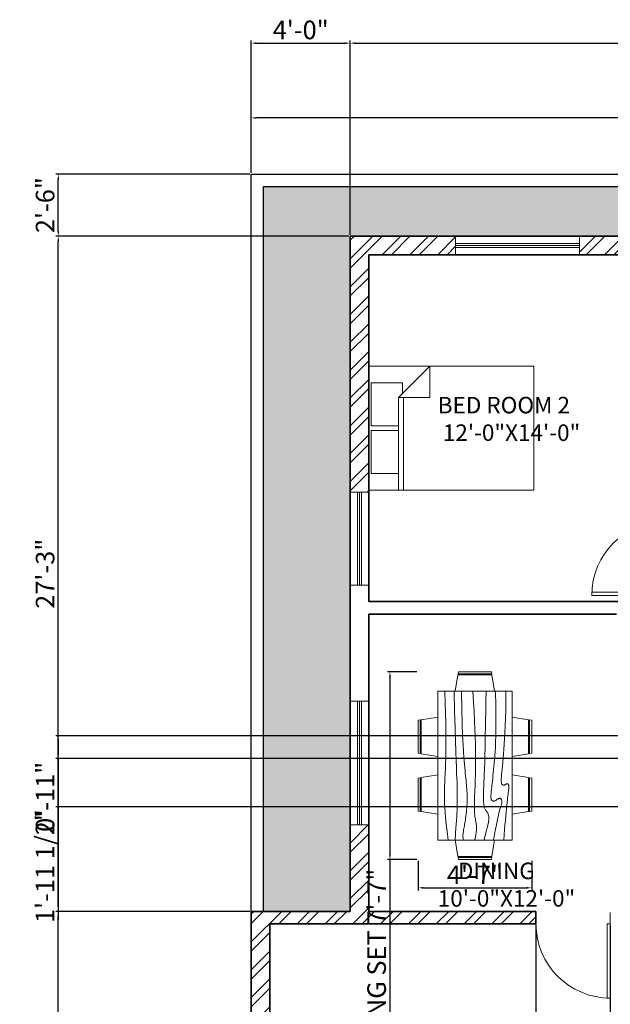
# Model space of a CAD drawing. Units: inches. Extents: x 108 to 883, y 608 to 1524.
# Tile 2 of 4: x 123 to 409, y 1040 to 1517. Entities that reach past the tile are written whole.
import ezdxf

# ---------------------------------------------------------------- set-up
doc = ezdxf.new("R2010")
doc.units = ezdxf.units.IN
for name, color, linetype, lineweight in [('A-ANNO-DIMS', 2, 'Continuous', 18), ('A-AREA-IDEN', 7, 'Continuous', 18), ('A-DOOR', 4, 'Continuous', 18), ('A-FURN', 8, 'Continuous', 18), ('A-WALL', 7, 'Continuous', 35), ('A-WALL-PATT', 252, 'Continuous', 13), ('C-PROP', 7, 'Continuous', 25)]:
    doc.layers.add(name, color=color, linetype=linetype, lineweight=lineweight)
doc.layers.add('A-GLAZ', color=244, linetype='Continuous', lineweight=18, true_color=0x991b1e)
doc.layers.add('L-PLNT-PATT', color=116, linetype='Continuous', lineweight=13, true_color=0x136734)
doc.styles.get("Standard").update_dxf_attribs({"font": 'arial.ttf'})
doc.dimstyles.new('ISO-25', dxfattribs={"dimtxt": 9, "dimasz": 2.5, "dimexe": 1.25, "dimexo": 0.625, "dimtad": 1, "dimlunit": 3, "dimtxsty": 'Standard', "dimcen": 2.5, "dimadec": 0, "dimazin": 0, "dimtfac": 1, "dimtmove": 0, "dimatfit": 3, "dimfxl": 1, "dimarcsym": 0})

# ---------------------------------------------------------------- blocks, each defined once
blk = doc.blocks.new('*U3')
for p, q in [((-40, 0), (-40, 6)), ((0, 0), (0, 6))]:
    blk.add_line(p, q)
blk.add_lwpolyline([(0, 0), (0, -40), (-1.75, -40), (-1.75, 0)], close=True)
blk.add_arc((0, 0), 40, 180, 270)
blk = doc.blocks.new('Bed - Queen')
for p, q in [((0, -80.00003), (0, 0)), ((0, 0), (59.99999, 0)), ((59.99999, 0), (59.99999, -80.00003)), ((7.99999, -1.2), (28.79998, -1.2)), ((7.99999, -14.4), (7.99999, -1.2)), ((28.79998, -1.2), (28.79998, -14.4)), ((31.19999, -1.2), (51.99999, -1.2)), ((31.19999, -14.4), (31.19999, -1.2)), ((51.99999, -1.2), (51.99999, -16.4)), ((0, -14.4), (44.8, -14.4)), ((44.8, -16.8), (0, -16.8)), ((59.99999, -29.6), (44.8, -14.4)), ((44.8, -14.4), (44.8, -29.6)), ((51.99999, -16.4), (46.79936, -16.4)), ((44.8, -29.6), (59.99999, -29.6)), ((59.99999, -80.00003), (0, -80.00003))]:
    blk.add_line(p, q)
blk = doc.blocks.new('Dining Set - 36 x 72 in.')
for p, q in [((-22.2343, 26.00059), (-23.4847, 17.99762)), ((-22.2304, 26), (-5.7608, 26)), ((-22, 27.5), (-22.1562, 26.50042)), ((-5.8416, 26.5), (-22.1534, 26.5)), ((-22, 27.5), (-6, 27.5)), ((-5.8437, 26.49966), (-6, 27.5)), ((-4.5152, 17.99762), (-5.7655, 25.99926)), ((5.7657, 26.00059), (4.5153, 17.99762)), ((5.7696, 26), (22.2392, 26)), ((6, 27.5), (5.8438, 26.50042)), ((22.1584, 26.5), (5.8466, 26.5)), ((6, 27.5), (22, 27.5)), ((22.1563, 26.49966), (22, 27.5)), ((23.4848, 17.99762), (22.2345, 25.99926)), ((36, 18), (-36, 18)), ((-36, 18), (-36, -18)), ((36, -18), (36, 18)), ((-45.5, 8), (-44.5004, 8.15617)), ((-45.5, 8), (-45.5, -8)), ((-44.5, -8.15843), (-44.5, 8.15338)), ((-44.0006, 8.23428), (-35.9976, 9.48474)), ((-44, 8.23041), (-44, -8.23915)), ((44.0006, 8.23428), (35.9976, 9.48474)), ((44, 8.23041), (44, -8.23915)), ((44.5, -8.15843), (44.5, 8.15338)), ((45.5, 8), (44.5005, 8.15617)), ((45.5, 8), (45.5, -8)), ((-44.4997, -8.15631), (-45.5, -8)), ((-35.9976, -9.48476), (-43.9993, -8.2345)), ((35.9976, -9.48476), (43.9993, -8.2345)), ((44.4997, -8.15631), (45.5, -8)), ((-36, -18), (36, -18)), ((-22.2343, -26.0006), (-23.4847, -17.99762)), ((-4.5152, -17.99762), (-5.7655, -25.99928)), ((5.7657, -26.0006), (4.5153, -17.99762)), ((23.4848, -17.99762), (22.2345, -25.99928)), ((-22.2304, -26), (-5.7608, -26)), ((-22, -27.5), (-22.1562, -26.50044)), ((-5.8416, -26.5), (-22.1534, -26.5)), ((-22, -27.5), (-6, -27.5)), ((-5.8437, -26.49967), (-6, -27.5)), ((5.7696, -26), (22.2392, -26)), ((6, -27.5), (5.8438, -26.50044)), ((22.1584, -26.5), (5.8466, -26.5)), ((6, -27.5), (22, -27.5)), ((22.1563, -26.49967), (22, -27.5))]:
    blk.add_line(p, q)
for points in [[(-36, 15), (-31.1772, 14.97754), (-26.8079, 14.91406), (-22.8538, 14.81543), (-19.276, 14.6875), (-16.0362, 14.53613), (-13.0957, 14.36718), (-10.4159, 14.18652), (-7.9583, 14), (-5.6904, 13.81315), (-3.6035, 13.63021), (-1.6954, 13.45508), (0.0365, 13.29166), (1.5945, 13.14388), (2.9811, 13.01562), (4.1988, 12.9108), (5.25, 12.83333), (6.1393, 12.78613), (6.8802, 12.76823), (7.4883, 12.77767), (7.9792, 12.8125), (8.3685, 12.87077), (8.6719, 12.95052), (8.9049, 13.0498), (9.0833, 13.16666), (9.2205, 13.29899), (9.3216, 13.44401), (9.3895, 13.59879), (9.4271, 13.76041), (9.4373, 13.92594), (9.4232, 14.09245), (9.3875, 14.257), (9.3333, 14.41666), (9.2638, 14.56917), (9.1836, 14.71484), (9.0975, 14.85465), (9.0104, 14.98958), (8.9272, 15.1206), (8.8529, 15.2487), (8.7922, 15.37483), (8.75, 15.5), (8.7305, 15.62467), (8.7344, 15.74739), (8.7617, 15.86621), (8.8125, 15.97916), (8.8867, 16.08431), (8.9844, 16.17968), (9.1055, 16.26334), (9.25, 16.33333), (9.4189, 16.38802), (9.6172, 16.42708), (9.8506, 16.45052), (10.125, 16.45833), (10.4463, 16.45052), (10.8203, 16.42708), (11.2529, 16.38802), (11.75, 16.33333), (12.3184, 16.26318), (12.9694, 16.17838), (13.7151, 16.07991), (14.5677, 15.96875), (15.5395, 15.84586), (16.6426, 15.71224), (17.8893, 15.56884), (19.2917, 15.41666), (20.859, 15.25667), (22.5879, 15.08984), (24.4721, 14.91715), (26.5052, 14.73958), (28.6809, 14.5581), (30.9929, 14.3737), (33.4347, 14.18733), (36, 14)], [(-36, 10), (-28.9766, 10.14274), (-23.1725, 10.20442), (-18.4241, 10.19775), (-14.5677, 10.13541), (-11.4399, 10.03011), (-8.877, 9.89453), (-6.7154, 9.74137), (-4.7917, 9.58333), (-2.9698, 9.43082), (-1.2246, 9.28515), (0.4415, 9.14534), (2.026, 9.01041), (3.5266, 8.87939), (4.9408, 8.7513), (6.266, 8.62516), (7.5, 8.5), (8.6411, 8.37549), (9.6914, 8.2539), (10.6538, 8.13818), (11.5312, 8.03125), (12.3267, 7.93603), (13.043, 7.85547), (13.6831, 7.79248), (14.25, 7.75), (14.7471, 7.7303), (15.1797, 7.73307), (15.5537, 7.75732), (15.875, 7.80208), (16.1494, 7.86637), (16.3828, 7.94922), (16.5811, 8.04964), (16.75, 8.16666), (16.8944, 8.29915), (17.0143, 8.44531), (17.1089, 8.60319), (17.1771, 8.77083), (17.218, 8.94629), (17.2305, 9.1276), (17.2137, 9.31282), (17.1667, 9.5), (17.0895, 9.6875), (16.987, 9.875), (16.8649, 10.0625), (16.7292, 10.25), (16.5856, 10.4375), (16.4401, 10.625), (16.2985, 10.8125), (16.1667, 11), (16.05, 11.18733), (15.9518, 11.3737), (15.8752, 11.5581), (15.8229, 11.73958), (15.798, 11.91715), (15.8034, 12.08984), (15.842, 12.25667), (15.9167, 12.41666), (16.0295, 12.56836), (16.1784, 12.70833), (16.3605, 12.83268), (16.5729, 12.9375), (16.8127, 13.01888), (17.0768, 13.07291), (17.3625, 13.0957), (17.6667, 13.08333), (17.9894, 13.03312), (18.3418, 12.94726), (18.7382, 12.82918), (19.1927, 12.68229), (19.7195, 12.51001), (20.3327, 12.31575), (21.0465, 12.10294), (21.875, 11.875), (22.8357, 11.63354), (23.959, 11.37304), (25.2786, 11.08618), (26.8282, 10.76562), (28.6414, 10.40405), (30.752, 9.99414), (33.1936, 9.52856), (36, 9)], [(-36, 5.5), (-30.7157, 5.3348), (-26.069, 5.20963), (-21.9946, 5.11767), (-18.4271, 5.05208), (-15.3009, 5.00602), (-12.5508, 4.97265), (-10.1112, 4.94515), (-7.9167, 4.91666), (-5.909, 4.88167), (-4.0586, 4.83984), (-2.3429, 4.79215), (-0.7396, 4.73958), (0.7739, 4.6831), (2.22, 4.6237), (3.6213, 4.56233), (5, 4.5), (6.373, 4.43782), (7.7344, 4.3776), (9.0723, 4.32129), (10.375, 4.27083), (11.6309, 4.22819), (12.8281, 4.19531), (13.9551, 4.17415), (15, 4.16666), (15.954, 4.17448), (16.819, 4.19791), (17.6001, 4.23698), (18.3021, 4.29166), (18.9299, 4.36198), (19.4883, 4.44791), (19.9823, 4.54948), (20.4167, 4.66666), (20.7969, 4.79899), (21.1302, 4.94401), (21.4245, 5.09879), (21.6875, 5.26041), (21.9271, 5.42594), (22.1511, 5.59245), (22.3672, 5.757), (22.5834, 5.91666), (22.8065, 6.06868), (23.0404, 6.21093), (23.2879, 6.34147), (23.5521, 6.45833), (23.8358, 6.55957), (24.142, 6.64323), (24.4735, 6.70735), (24.8334, 6.75), (25.2235, 6.76969), (25.642, 6.76692), (26.0858, 6.74267), (26.5521, 6.69791), (27.0379, 6.63362), (27.5404, 6.55078), (28.0565, 6.45036), (28.5834, 6.33333), (29.1242, 6.19987), (29.7071, 6.04687), (30.3661, 5.87044), (31.1354, 5.66666), (32.0493, 5.43164), (33.142, 5.16146), (34.4475, 4.85221), (36, 4.5)], [(-36, -1), (-30.7915, -0.6591), (-26.0195, -0.38216), (-21.6519, -0.16284), (-17.6563, 0.00521), (-14.0005, 0.12833), (-10.6523, 0.21289), (-7.5796, 0.26522), (-4.75, 0.29166), (-2.134, 0.29793), (0.2878, 0.28711), (2.5317, 0.26163), (4.6146, 0.22396), (6.5529, 0.17651), (8.3633, 0.12174), (10.0623, 0.06209), (11.6667, 0), (13.1899, -0.06201), (14.6341, -0.1211), (15.9982, -0.17432), (17.2813, -0.21875), (18.4823, -0.25147), (19.6003, -0.26953), (20.6343, -0.27002), (21.5834, -0.25), (22.4481, -0.20768), (23.2357, -0.14584), (23.9549, -0.06836), (24.6146, 0.02083), (25.2235, 0.11784), (25.7904, 0.21875), (26.3241, 0.31966), (26.8334, 0.41666), (27.3265, 0.50618), (27.8099, 0.58593), (28.2894, 0.65397), (28.7709, 0.70833), (29.2601, 0.74707), (29.763, 0.76823), (30.2855, 0.76985), (30.8334, 0.75), (31.4088, 0.70784), (31.9994, 0.64713), (32.589, 0.57275), (33.1615, 0.48958), (33.7008, 0.4025), (34.1908, 0.3164), (34.6153, 0.23616), (34.9584, 0.16666), (35.2099, 0.11165), (35.3848, 0.07031), (35.504, 0.04069), (35.5886, 0.02083), (35.6594, 0.00879), (35.7377, 0.0026), (35.8442, 0.00032), (36, 0)], [(-36, -6.5), (-27.1843, -6.31267), (-20.084, -6.1263), (-14.469, -5.9419), (-10.1094, -5.76042), (-6.7752, -5.58285), (-4.2363, -5.41016), (-2.2629, -5.24333), (-0.625, -5.08334), (0.8708, -4.93099), (2.2715, -4.78646), (3.5872, -4.64974), (4.8281, -4.52084), (6.0046, -4.39974), (7.127, -4.28646), (8.2053, -4.18099), (9.25, -4.08334), (10.2705, -3.99382), (11.2734, -3.91407), (12.2647, -3.84603), (13.25, -3.79167), (14.2354, -3.75293), (15.2266, -3.73177), (16.2295, -3.73015), (17.25, -3.75), (18.2912, -3.79248), (19.3451, -3.85547), (20.4009, -3.93604), (21.4479, -4.03125), (22.4754, -4.13819), (23.4727, -4.25391), (24.4289, -4.37549), (25.3334, -4.5), (26.1785, -4.62492), (26.9694, -4.74935), (27.7145, -4.87281), (28.4219, -4.99479), (29.1, -5.11483), (29.7572, -5.23242), (30.4016, -5.34709), (31.0417, -5.45834), (31.6837, -5.56437), (32.3262, -5.65821), (32.9658, -5.73153), (33.599, -5.77604), (34.2224, -5.78345), (34.8327, -5.74545), (35.4264, -5.65373), (36, -5.5)], [(-36, -10), (-26.4022, -9.81299), (-18.4675, -9.62891), (-11.9839, -9.45069), (-6.7396, -9.28125), (-2.5226, -9.12354), (0.8789, -8.98047), (3.6769, -8.85498), (6.0833, -8.75), (8.2767, -8.66765), (10.3021, -8.60677), (12.1712, -8.56543), (13.8958, -8.54167), (15.4876, -8.53353), (16.9583, -8.53907), (18.3197, -8.55632), (19.5834, -8.58334), (20.7616, -8.61841), (21.8685, -8.66081), (22.9188, -8.71004), (23.9271, -8.76563), (24.9081, -8.82707), (25.8763, -8.89388), (26.8465, -8.96558), (27.8334, -9.04167), (28.8474, -9.12118), (29.8828, -9.20117), (30.93, -9.27824), (31.9792, -9.34896), (33.0205, -9.40991), (34.0443, -9.45768), (35.0407, -9.48885), (36, -9.5)], [(-36, -14.5), (-30.0881, -14.33513), (-25.0332, -14.21224), (-20.7312, -14.12647), (-17.0781, -14.07292), (-13.97, -14.04671), (-11.3027, -14.04297), (-8.9724, -14.05681), (-6.875, -14.08334), (-4.9224, -14.11833), (-3.0905, -14.16016), (-1.3709, -14.20785), (0.2448, -14.26042), (1.7647, -14.3169), (3.1973, -14.3763), (4.5507, -14.43767), (5.8333, -14.5), (7.0554, -14.5621), (8.235, -14.62175), (9.3922, -14.67652), (10.5469, -14.72396), (11.7192, -14.76164), (12.929, -14.78711), (14.1965, -14.79794), (15.5417, -14.79167), (16.9933, -14.76424), (18.6152, -14.70508), (20.4804, -14.60197), (22.6615, -14.44271), (25.2312, -14.21509), (28.2624, -13.9069), (31.8277, -13.50594), (36, -13)]]:
    blk.add_lwpolyline(points)
blk = doc.blocks.new('*D15')
at = {"layer": 'A-ANNO-DIMS', "color": 0, "lineweight": -2, "transparency": 16777216}
for p, q in [((235.21, 1442.8), (235.21, 1470.67)), ((754.62, 1469.42), (237.71, 1469.42)), ((757.12, 1442.8), (757.12, 1470.67))]:
    blk.add_line(p, q, dxfattribs=at)
at = {"layer": 'A-ANNO-DIMS', "color": 0, "transparency": 16777216}
for points in [[(237.71, 1469.84), (237.71, 1469.01), (235.21, 1469.42)], [(754.62, 1469.84), (754.62, 1469.01), (757.12, 1469.42)]]:
    blk.add_solid(points, dxfattribs=at)
at = {"layer": 'Defpoints', "color": 0, "transparency": 16777216}
for p in [(235.21, 1469.42), (235.21, 1442.18), (757.12, 1442.18)]:
    blk.add_point(p, dxfattribs=at)
at = {"layer": 'A-ANNO-DIMS', "color": 0, "transparency": 16777216, "insert": (496.17, 1474.65), "char_height": 9, "attachment_point": 5}
blk.add_mtext('43\'-5.91"', dxfattribs=at)
blk = doc.blocks.new('WIN-45IN-EXT')
for p, q in [((3.5, 45), (3.5, 0)), ((4.5, 45), (4.5, 0)), ((5.5, 45), (5.5, 0))]:
    blk.add_line(p, q)
blk.add_lwpolyline([(9, 45), (9, 0), (0, 0), (0, 45)], close=True)
blk = doc.blocks.new('WIN-60IN-EXT')
for p, q in [((60, 5.5), (0, 5.5)), ((60, 4.5), (0, 4.5)), ((60, 3.5), (0, 3.5))]:
    blk.add_line(p, q)
blk.add_lwpolyline([(60, 9), (60, 0), (0, 0), (0, 9)], close=True)
blk = doc.blocks.new('*D42')
at = {"layer": 'A-ANNO-DIMS', "color": 0, "lineweight": -2, "transparency": 16777216}
for p, q in [((315.42, 1201.24), (301.14, 1201.24)), ((302.39, 1198.74), (302.39, 1112.74)), ((315.42, 1110.24), (301.14, 1110.24)), ((302.39, 1110.24), (302.39, 1007.57))]:
    blk.add_line(p, q, dxfattribs=at)
at = {"layer": 'A-ANNO-DIMS', "color": 0, "transparency": 16777216}
for points in [[(301.98, 1198.74), (302.81, 1198.74), (302.39, 1201.24)], [(301.98, 1112.74), (302.81, 1112.74), (302.39, 1110.24)]]:
    blk.add_solid(points, dxfattribs=at)
at = {"layer": 'Defpoints', "color": 0, "transparency": 16777216}
for p in [(316.04, 1201.24), (302.39, 1110.24), (316.04, 1110.24)]:
    blk.add_point(p, dxfattribs=at)
at = {"layer": 'A-ANNO-DIMS', "color": 0, "transparency": 16777216, "insert": (297.11, 1057.66), "char_height": 9, "attachment_point": 5, "rotation": 90}
blk.add_mtext('DINING SET 7\'-7"', dxfattribs=at)
blk = doc.blocks.new('*D43')
at = {"layer": 'A-ANNO-DIMS', "color": 0, "lineweight": -2, "transparency": 16777216}
for p, q in [((316.04, 1109.62), (316.04, 1095.34)), ((371.04, 1109.62), (371.04, 1095.34)), ((318.54, 1096.59), (368.54, 1096.59))]:
    blk.add_line(p, q, dxfattribs=at)
at = {"layer": 'A-ANNO-DIMS', "color": 0, "transparency": 16777216}
for points in [[(318.54, 1097.01), (318.54, 1096.18), (316.04, 1096.59)], [(368.54, 1097.01), (368.54, 1096.18), (371.04, 1096.59)]]:
    blk.add_solid(points, dxfattribs=at)
at = {"layer": 'Defpoints', "color": 0, "transparency": 16777216}
for p in [(316.04, 1110.24), (371.04, 1110.24), (371.04, 1096.59)]:
    blk.add_point(p, dxfattribs=at)
at = {"layer": 'A-ANNO-DIMS', "color": 0, "transparency": 16777216, "insert": (343.54, 1101.72), "char_height": 9, "attachment_point": 5}
blk.add_mtext('4\'-7"', dxfattribs=at)
blk = doc.blocks.new('*D44')
at = {"layer": 'A-ANNO-DIMS', "color": 0, "lineweight": -2, "transparency": 16777216}
for p, q in [((283.12, 1412.8), (283.12, 1506.88)), ((727.12, 1412.8), (727.12, 1506.88)), ((285.62, 1505.63), (724.62, 1505.63))]:
    blk.add_line(p, q, dxfattribs=at)
at = {"layer": 'A-ANNO-DIMS', "color": 0, "transparency": 16777216}
for points in [[(285.62, 1506.04), (285.62, 1505.21), (283.12, 1505.63)], [(724.62, 1506.04), (724.62, 1505.21), (727.12, 1505.63)]]:
    blk.add_solid(points, dxfattribs=at)
at = {"layer": 'Defpoints', "color": 0, "transparency": 16777216}
for p in [(727.12, 1505.63), (283.12, 1412.18), (727.12, 1412.18)]:
    blk.add_point(p, dxfattribs=at)
at = {"layer": 'A-ANNO-DIMS', "color": 0, "transparency": 16777216, "insert": (505.12, 1510.85), "char_height": 9, "attachment_point": 5}
blk.add_mtext('37\'-0"', dxfattribs=at)
blk = doc.blocks.new('*D45')
at = {"layer": 'A-ANNO-DIMS', "color": 0, "lineweight": -2, "transparency": 16777216}
for p, q in [((234.59, 1442.18), (140.51, 1442.18)), ((141.76, 1414.68), (141.76, 1439.68)), ((282.5, 1412.18), (140.51, 1412.18))]:
    blk.add_line(p, q, dxfattribs=at)
at = {"layer": 'A-ANNO-DIMS', "color": 0, "transparency": 16777216}
for points in [[(141.35, 1439.68), (142.18, 1439.68), (141.76, 1442.18)], [(141.35, 1414.68), (142.18, 1414.68), (141.76, 1412.18)]]:
    blk.add_solid(points, dxfattribs=at)
at = {"layer": 'Defpoints', "color": 0, "transparency": 16777216}
for p in [(141.76, 1442.18), (235.21, 1442.18), (283.12, 1412.18)]:
    blk.add_point(p, dxfattribs=at)
at = {"layer": 'A-ANNO-DIMS', "color": 0, "transparency": 16777216, "insert": (136.54, 1427.18), "char_height": 9, "attachment_point": 5, "rotation": 90}
blk.add_mtext('2\'-6"', dxfattribs=at)
blk = doc.blocks.new('*D47')
at = {"layer": 'A-ANNO-DIMS', "color": 0, "lineweight": -2, "transparency": 16777216}
for p, q in [((235.21, 1442.8), (235.21, 1506.88)), ((283.12, 1412.8), (283.12, 1506.88)), ((237.71, 1505.63), (280.62, 1505.63))]:
    blk.add_line(p, q, dxfattribs=at)
at = {"layer": 'A-ANNO-DIMS', "color": 0, "transparency": 16777216}
for points in [[(237.71, 1506.04), (237.71, 1505.21), (235.21, 1505.63)], [(280.62, 1506.04), (280.62, 1505.21), (283.12, 1505.63)]]:
    blk.add_solid(points, dxfattribs=at)
at = {"layer": 'Defpoints', "color": 0, "transparency": 16777216}
for p in [(283.12, 1505.63), (235.21, 1442.18), (283.12, 1412.18)]:
    blk.add_point(p, dxfattribs=at)
at = {"layer": 'A-ANNO-DIMS', "color": 0, "transparency": 16777216, "insert": (259.17, 1510.85), "char_height": 9, "attachment_point": 5}
blk.add_mtext('4\'-0"', dxfattribs=at)
blk = doc.blocks.new('*D49')
at = {"layer": 'A-ANNO-DIMS', "color": 0, "lineweight": -2, "transparency": 16777216}
for p, q in [((234.59, 1085.18), (140.51, 1085.18)), ((141.76, 778.68), (141.76, 1082.68)), ((234.59, 776.18), (140.51, 776.18))]:
    blk.add_line(p, q, dxfattribs=at)
at = {"layer": 'A-ANNO-DIMS', "color": 0, "transparency": 16777216}
for points in [[(141.35, 1082.68), (142.18, 1082.68), (141.76, 1085.18)], [(141.35, 778.68), (142.18, 778.68), (141.76, 776.18)]]:
    blk.add_solid(points, dxfattribs=at)
at = {"layer": 'Defpoints', "color": 0, "transparency": 16777216}
for p in [(141.76, 1085.18), (235.21, 1085.18), (235.21, 776.18)]:
    blk.add_point(p, dxfattribs=at)
at = {"layer": 'A-ANNO-DIMS', "color": 0, "transparency": 16777216, "insert": (136.54, 930.68), "char_height": 9, "attachment_point": 5, "rotation": 90}
blk.add_mtext('25\'-9"', dxfattribs=at)
blk = doc.blocks.new('*D50')
at = {"layer": 'A-ANNO-DIMS', "color": 0, "lineweight": -2, "transparency": 16777216}
for p, q in [((282.5, 1412.18), (140.51, 1412.18)), ((141.76, 1087.68), (141.76, 1409.68)), ((234.59, 1085.18), (140.51, 1085.18))]:
    blk.add_line(p, q, dxfattribs=at)
at = {"layer": 'A-ANNO-DIMS', "color": 0, "transparency": 16777216}
for points in [[(141.35, 1409.68), (142.18, 1409.68), (141.76, 1412.18)], [(141.35, 1087.68), (142.18, 1087.68), (141.76, 1085.18)]]:
    blk.add_solid(points, dxfattribs=at)
at = {"layer": 'Defpoints', "color": 0, "transparency": 16777216}
for p in [(141.76, 1412.18), (283.12, 1412.18), (235.21, 1085.18)]:
    blk.add_point(p, dxfattribs=at)
at = {"layer": 'A-ANNO-DIMS', "color": 0, "transparency": 16777216, "insert": (136.54, 1248.68), "char_height": 9, "attachment_point": 5, "rotation": 90}
blk.add_mtext('27\'-3"', dxfattribs=at)
blk = doc.blocks.new('*D51')
at = {"layer": 'A-ANNO-DIMS', "color": 0, "lineweight": -2, "transparency": 16777216}
for p, q in [((373.12, 1078.55), (373.12, 608.47)), ((409.12, 1078.55), (409.12, 608.47)), ((375.62, 609.72), (406.62, 609.72))]:
    blk.add_line(p, q, dxfattribs=at)
at = {"layer": 'A-ANNO-DIMS', "color": 0, "transparency": 16777216}
for points in [[(375.62, 610.13), (375.62, 609.3), (373.12, 609.72)], [(406.62, 610.13), (406.62, 609.3), (409.12, 609.72)]]:
    blk.add_solid(points, dxfattribs=at)
at = {"layer": 'Defpoints', "color": 0, "transparency": 16777216}
for p in [(373.12, 1079.18), (409.12, 1079.18), (409.12, 609.72)]:
    blk.add_point(p, dxfattribs=at)
at = {"layer": 'A-ANNO-DIMS', "color": 0, "transparency": 16777216, "insert": (391.12, 614.94), "char_height": 9, "attachment_point": 5}
blk.add_mtext('3\'-0"', dxfattribs=at)
blk = doc.blocks.new('*D56')
at = {"layer": 'A-ANNO-DIMS', "color": 0, "lineweight": -2, "transparency": 16777216}
for p, q in [((705.55, 1159.23), (140.51, 1159.23)), ((141.76, 1156.73), (141.76, 1138.26)), ((705.55, 1135.76), (140.51, 1135.76)), ((141.76, 1135.76), (141.76, 1080.97))]:
    blk.add_line(p, q, dxfattribs=at)
at = {"layer": 'A-ANNO-DIMS', "color": 0, "transparency": 16777216}
for points in [[(141.35, 1156.73), (142.18, 1156.73), (141.76, 1159.23)], [(141.35, 1138.26), (142.18, 1138.26), (141.76, 1135.76)]]:
    blk.add_solid(points, dxfattribs=at)
at = {"layer": 'Defpoints', "color": 0, "transparency": 16777216}
for p in [(706.17, 1159.23), (141.76, 1135.76), (706.17, 1135.76)]:
    blk.add_point(p, dxfattribs=at)
at = {"layer": 'A-ANNO-DIMS', "color": 0, "transparency": 16777216, "insert": (136.48, 1107.11), "char_height": 9, "attachment_point": 5, "rotation": 90}
blk.add_mtext('1\'-11 1/2"', dxfattribs=at)
blk = doc.blocks.new('*D57')
at = {"layer": 'A-ANNO-DIMS', "color": 0, "lineweight": -2, "transparency": 16777216}
for p, q in [((694.94, 1170.23), (140.51, 1170.23)), ((141.76, 1167.73), (141.76, 1161.73)), ((705.55, 1159.23), (140.51, 1159.23)), ((141.76, 1159.23), (141.76, 1124.56))]:
    blk.add_line(p, q, dxfattribs=at)
at = {"layer": 'A-ANNO-DIMS', "color": 0, "transparency": 16777216}
for points in [[(141.35, 1167.73), (142.18, 1167.73), (141.76, 1170.23)], [(141.35, 1161.73), (142.18, 1161.73), (141.76, 1159.23)]]:
    blk.add_solid(points, dxfattribs=at)
at = {"layer": 'Defpoints', "color": 0, "transparency": 16777216}
for p in [(695.57, 1170.23), (141.76, 1159.23), (706.17, 1159.23)]:
    blk.add_point(p, dxfattribs=at)
at = {"layer": 'A-ANNO-DIMS', "color": 0, "transparency": 16777216, "insert": (136.54, 1140.64), "char_height": 9, "attachment_point": 5, "rotation": 90}
blk.add_mtext('0\'-11"', dxfattribs=at)

msp = doc.modelspace()

# ---------------------------------------------------------------- hatches: boundary and pattern name
at = {"layer": 'A-WALL-PATT'}
h = msp.add_hatch(dxfattribs=at)
h.set_pattern_fill('ANSI32', color=256)
h.paths.add_polyline_path([(373.121, 1085.177), (292.121, 1085.177), (292.121, 1127.011), (283.121, 1127.011), (283.121, 1085.177), (235.212, 1085.177), (235.212, 1029.423), (244.212, 1029.423), (244.212, 1079.177), (373.121, 1079.177), (373.121, 1084.577)])
h.paths.add_polyline_path([(349.212, 911.177), (244.212, 911.177), (244.212, 969.423), (235.212, 969.423), (235.212, 776.177), (266.885, 776.177), (266.885, 785.177), (244.212, 785.177), (244.212, 905.177), (316.212, 905.177), (316.212, 902.177), (322.212, 902.177), (322.212, 905.177), (349.212, 905.177)])
h.paths.add_polyline_path([(484.212, 839.177), (473.778, 839.177), (473.778, 830.177), (478.212, 830.177), (478.212, 770.177), (484.212, 770.177), (484.212, 801.677), (490.212, 801.677), (490.212, 806.177), (490.212, 807.677), (484.212, 807.677)])
h.paths.add_polyline_path([(562.212, 830.177), (566.671, 830.177), (566.671, 839.177), (556.212, 839.177), (556.212, 807.677), (550.212, 807.677), (550.212, 806.177), (550.212, 801.677), (556.212, 801.677), (556.212, 770.177), (562.212, 770.177)])
h.paths.add_polyline_path([(622.212, 848.109), (613.212, 848.109), (613.212, 839.177), (611.671, 839.177), (611.671, 830.177), (622.212, 830.177)])
h.paths.add_polyline_path([(690.201, 911.177), (619.212, 911.177), (619.212, 1031.177), (653.667, 1031.177), (653.667, 1037.177), (613.212, 1037.177), (613.212, 893.109), (622.212, 893.109), (622.212, 902.177), (690.201, 902.177)])
h.paths.add_polyline_path([(727.121, 941.177), (718.121, 941.177), (718.121, 911.177), (711.201, 911.177), (711.201, 902.177), (727.121, 902.177)])
h.paths.add_polyline_path([(727.121, 1103.177), (718.121, 1103.177), (718.121, 1037.177), (683.667, 1037.177), (683.667, 1031.177), (718.121, 1031.177), (718.121, 1001.177), (727.121, 1001.177)])
h.paths.add_polyline_path([(727.121, 1412.177), (676.121, 1412.177), (676.121, 1403.177), (718.121, 1403.177), (718.121, 1295.236), (727.121, 1295.236)])
h.paths.add_polyline_path([(574.121, 1403.177), (616.121, 1403.177), (616.121, 1412.177), (548.621, 1412.177), (548.621, 1403.177), (568.121, 1403.177), (568.121, 1307.177), (565.121, 1307.177), (565.121, 1301.177), (568.121, 1301.177), (568.121, 1274.177), (574.121, 1274.177)])
h.paths.add_polyline_path([(508.121, 1403.177), (527.621, 1403.177), (527.621, 1412.177), (483.029, 1412.177), (483.029, 1403.177), (502.121, 1403.177), (502.121, 1307.177), (475.121, 1307.177), (475.121, 1301.177), (535.121, 1301.177), (535.121, 1307.177), (508.121, 1307.177)])
h.paths.add_polyline_path([(462.029, 1412.177), (394.121, 1412.177), (394.121, 1403.177), (436.121, 1403.177), (436.121, 1274.177), (442.121, 1274.177), (442.121, 1301.177), (445.121, 1301.177), (445.121, 1307.177), (442.121, 1307.177), (442.121, 1403.177), (462.029, 1403.177)])
h.paths.add_polyline_path([(334.121, 1412.177), (283.121, 1412.177), (283.121, 1288.13), (292.121, 1288.13), (292.121, 1403.177), (334.121, 1403.177)])
at = {"layer": 'L-PLNT-PATT'}
h = msp.add_hatch(dxfattribs=at)
h.set_pattern_fill('CROSS', color=256)
h.paths.add_polyline_path([(751.121, 1436.177), (241.212, 1436.177), (241.212, 1085.177), (283.121, 1085.177), (283.121, 1412.177), (727.121, 1412.177), (727.121, 902.177), (751.121, 902.177)])

# ---------------------------------------------------------------- linework, layer by layer
at = {"layer": 'A-WALL'}
for p, q in [((283.121, 1412.177), (283.121, 1085.177)), ((283.121, 1412.177), (727.121, 1412.177)), ((292.121, 1403.177), (292.121, 1235.177)), ((292.121, 1403.177), (436.121, 1403.177)), ((292.121, 1235.177), (436.121, 1235.177)), ((292.121, 1229.177), (412.121, 1229.177)), ((292.121, 1229.177), (292.121, 1085.177)), ((235.212, 1085.177), (283.121, 1085.177)), ((235.212, 1085.177), (235.212, 776.177)), ((292.121, 1085.177), (373.121, 1085.177)), ((373.121, 1085.177), (373.121, 1079.177)), ((244.212, 1079.177), (373.121, 1079.177)), ((244.212, 1079.177), (244.212, 911.177))]:
    msp.add_line(p, q, dxfattribs=at)
at = {"layer": 'C-PROP'}
for p, q in [((235.212, 1085.177), (235.212, 1442.177)), ((235.212, 1442.177), (757.121, 1442.177)), ((241.212, 1085.177), (241.212, 1436.177)), ((241.212, 1436.177), (751.121, 1436.177))]:
    msp.add_line(p, q, dxfattribs=at)

# ---------------------------------------------------------------- block references
at = {"layer": 'A-DOOR', "xscale": 0.8999869424387545, "yscale": 0.8999869424387545, "zscale": 0.8999869424387545, "rotation": 270}
msp.add_blockref('*U3', (436.121, 1238.177), dxfattribs=at)
at = {"layer": 'A-DOOR', "xscale": 0.8999869424387545, "yscale": 0.8999869424387545, "zscale": 0.8999869424387545}
msp.add_blockref('*U3', (409.121, 1079.177), dxfattribs=at)
at = {"layer": 'A-FURN'}
for name, p, rotation in [('Bed - Queen', (292.121, 1289.177), 90), ('Dining Set - 36 x 72 in.', (343.543, 1155.742), 270)]:
    msp.add_blockref(name, p, dxfattribs=dict(at, rotation=rotation))
at = {"layer": 'A-GLAZ'}
for name, p in [('WIN-60IN-EXT', (334.121, 1403.177)), ('WIN-45IN-EXT', (283.122, 1243.13))]:
    msp.add_blockref(name, p, dxfattribs=at)
at = {"layer": 'A-GLAZ', "rotation": 90}
msp.add_blockref('WIN-60IN-EXT', (292.121, 1127.011), dxfattribs=at)

# ---------------------------------------------------------------- texts
at = {"layer": 'A-AREA-IDEN', "char_height": 8, "attachment_point": 1}
for s, width, insert in [('BED ROOM 2\\P 12\'-0"X14\'-0"', 70.1831, (325.543, 1334.334)), ('    DINING 10\'-0"X12\'-0"', 63.08794, (325.543, 1108.802))]:
    msp.add_mtext_dynamic_manual_height_columns(s, width=width, gutter_width=12.5, heights=[0], dxfattribs=dict(at, insert=insert))

# ---------------------------------------------------------------- dimensions: what is measured, and where the dimension line sits
at = {"layer": 'A-ANNO-DIMS'}
for base, p1, p2, override, picture, middle in [((283.121, 1505.627), (235.212, 1442.177), (283.121, 1412.177), {"dimdec": 1, "dimlfac": 1, "dimrnd": 0, "dimzin": 1, "dimdsep": 46, "dimlunit": 4, "dimfrac": 2}, '*D47', (259.167, 1510.847)), ((727.121, 1505.627), (283.121, 1412.177), (727.121, 1412.177), {"dimdec": 1, "dimlfac": 1, "dimrnd": 0, "dimzin": 1, "dimdsep": 46, "dimlunit": 4, "dimfrac": 2}, '*D44', (505.121, 1510.85)), ((235.212, 1469.422), (757.121, 1442.177), (235.212, 1442.177), {"dimclrd": 0, "dimclre": 0, "dimclrt": 0}, '*D15', (496.167, 1474.645)), ((371.043, 1096.592), (316.043, 1110.242), (371.043, 1110.242), {"dimdec": 1, "dimlfac": 1, "dimrnd": 0, "dimzin": 1, "dimdsep": 46, "dimlunit": 4, "dimfrac": 2}, '*D43', (343.543, 1101.717)), ((409.121, 609.715), (373.121, 1079.177), (409.121, 1079.177), {"dimdec": 1, "dimlfac": 1, "dimrnd": 0, "dimzin": 1, "dimdsep": 46, "dimlunit": 4, "dimfrac": 2}, '*D51', (391.121, 614.938))]:
    dim = msp.add_linear_dim(base=base, p1=p1, p2=p2, dimstyle='ISO-25', override=override, dxfattribs=at)
    dim.commit()
    dim.dimension.update_dxf_attribs({"geometry": picture, "text_midpoint": middle})
for base, p1, p2, picture, middle in [((141.762, 1442.177), (283.121, 1412.177), (235.212, 1442.177), '*D45', (136.542, 1427.177)), ((141.762, 1412.177), (235.212, 1085.177), (283.121, 1412.177), '*D50', (136.539, 1248.677)), ((141.762, 1159.227), (695.567, 1170.227), (706.173, 1159.227), '*D57', (136.542, 1140.644)), ((141.762, 1135.76), (706.173, 1159.227), (706.173, 1135.76), '*D56', (136.483, 1107.115)), ((141.762, 1085.177), (235.212, 776.177), (235.212, 1085.177), '*D49', (136.542, 930.677))]:
    dim = msp.add_linear_dim(base=base, p1=p1, p2=p2, angle=90, dimstyle='ISO-25', override={"dimdec": 1, "dimlfac": 1, "dimrnd": 0, "dimzin": 1, "dimdsep": 46, "dimlunit": 4, "dimfrac": 2}, dxfattribs=at)
    dim.commit()
    dim.dimension.update_dxf_attribs({"geometry": picture, "text_midpoint": middle})
dim = msp.add_linear_dim(base=(302.393, 1110.242), p1=(316.043, 1201.242), p2=(316.043, 1110.242), angle=270, text='DINING SET <>', dimstyle='ISO-25', override={"dimdec": 1, "dimlfac": 1, "dimrnd": 0, "dimzin": 1, "dimdsep": 46, "dimlunit": 4, "dimfrac": 2}, dxfattribs=at)
dim.commit()
dim.dimension.update_dxf_attribs({"geometry": '*D42', "text_midpoint": (297.114, 1057.657)})

doc.saveas('drawing.dxf')
